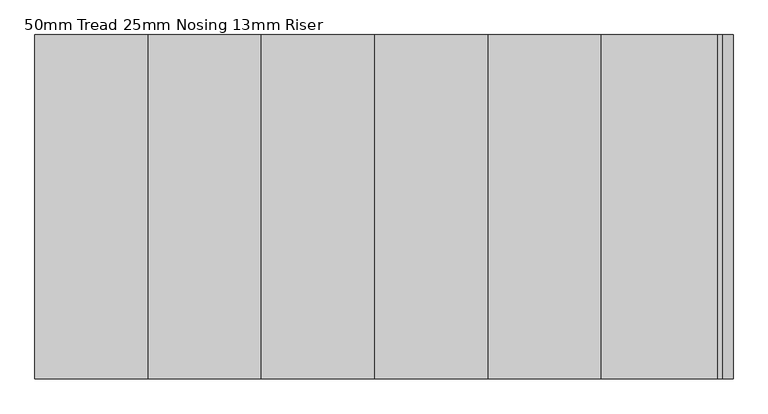
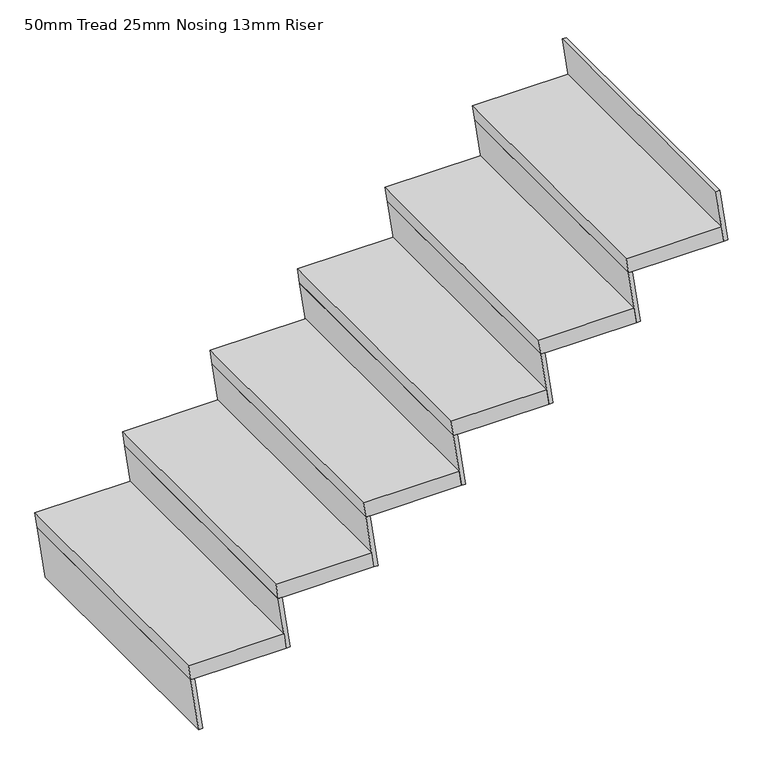
"""IFC4 building model written with IfcOpenShell, lengths in millimetres: stair flight geometry, 50mm Tread 25mm Nosing 13mm Riser."""

from ifc_helpers import new_model, si_unit, frame, origin, place, context, project, spatial, polyline, outline, extrude, source, transform, mapped, element, save


def stair_flight_50mm_tread_25mm_nosing_13mm_riser_89ce4123(model_context):
    return source(origin(), model_context, "Body", "SweptSolid", [
        extrude(outline(polyline([(1739.1304348, -8778.6870075), (1739.1304348, -9078.6870075), (1689.1304348, -9071.4995075), (1689.1304348, -8771.4995075), (1739.1304348, -8778.6870075)])), frame((0.0, 2408.8252453, 0.0), z_axis=(0.0, 1.0, 0.0), x_axis=(0.0, 0.0, 1.0)), (0.0, 0.0, 1.0), 835.4613281),
        extrude(outline(polyline([(1689.1304348, -9071.4995075), (1515.2173913, -9046.4995075), (1515.2173913, -9033.8710175), (1689.1304348, -9058.8710175), (1689.1304348, -9071.4995075)])), frame((0.0, 2408.8252453, 0.0), z_axis=(0.0, 1.0, 0.0), x_axis=(0.0, 0.0, 1.0)), (0.0, 0.0, 1.0), 835.4613281),
        extrude(outline(polyline([(1863.0434783, -8796.4995075), (1689.1304348, -8771.4995075), (1689.1304348, -8758.8710175), (1863.0434783, -8783.8710175), (1863.0434783, -8796.4995075)])), frame((0.0, 2408.8252453, 0.0), z_axis=(0.0, 1.0, 0.0), x_axis=(0.0, 0.0, 1.0)), (0.0, 0.0, 1.0), 835.4613281),
        extrude(outline(polyline([(1913.0434783, -8503.6870075), (1913.0434783, -8803.6870075), (1863.0434783, -8796.4995075), (1863.0434783, -8496.4995075), (1913.0434783, -8503.6870075)])), frame((0.0, 2408.8252453, 0.0), z_axis=(0.0, 1.0, 0.0), x_axis=(0.0, 0.0, 1.0)), (0.0, 0.0, 1.0), 835.4613281),
        extrude(outline(polyline([(2036.9565217, -8521.4995075), (1863.0434783, -8496.4995075), (1863.0434783, -8483.8710175), (2036.9565217, -8508.8710175), (2036.9565217, -8521.4995075)])), frame((0.0, 2408.8252453, 0.0), z_axis=(0.0, 1.0, 0.0), x_axis=(0.0, 0.0, 1.0)), (0.0, 0.0, 1.0), 835.4613281),
        extrude(outline(polyline([(2086.9565217, -8228.6870075), (2086.9565217, -8528.6870075), (2036.9565217, -8521.4995075), (2036.9565217, -8221.4995075), (2086.9565217, -8228.6870075)])), frame((0.0, 2408.8252453, 0.0), z_axis=(0.0, 1.0, 0.0), x_axis=(0.0, 0.0, 1.0)), (0.0, 0.0, 1.0), 835.4613281),
        extrude(outline(polyline([(2210.8695652, -8246.4995075), (2036.9565217, -8221.4995075), (2036.9565217, -8208.8710175), (2210.8695652, -8233.8710175), (2210.8695652, -8246.4995075)])), frame((0.0, 2408.8252453, 0.0), z_axis=(0.0, 1.0, 0.0), x_axis=(0.0, 0.0, 1.0)), (0.0, 0.0, 1.0), 835.4613281),
        extrude(outline(polyline([(2260.8695652, -7953.6870075), (2260.8695652, -8253.6870075), (2210.8695652, -8246.4995075), (2210.8695652, -7946.4995075), (2260.8695652, -7953.6870075)])), frame((0.0, 2408.8252453, 0.0), z_axis=(0.0, 1.0, 0.0), x_axis=(0.0, 0.0, 1.0)), (0.0, 0.0, 1.0), 835.4613281),
        extrude(outline(polyline([(2384.7826087, -7971.4995075), (2210.8695652, -7946.4995075), (2210.8695652, -7933.8710175), (2384.7826087, -7958.8710175), (2384.7826087, -7971.4995075)])), frame((0.0, 2408.8252453, 0.0), z_axis=(0.0, 1.0, 0.0), x_axis=(0.0, 0.0, 1.0)), (0.0, 0.0, 1.0), 835.4613281),
        extrude(outline(polyline([(2434.7826087, -7678.6870075), (2434.7826087, -7978.6870075), (2384.7826087, -7971.4995075), (2384.7826087, -7671.4995075), (2434.7826087, -7678.6870075)])), frame((0.0, 2408.8252453, 0.0), z_axis=(0.0, 1.0, 0.0), x_axis=(0.0, 0.0, 1.0)), (0.0, 0.0, 1.0), 835.4613281),
        extrude(outline(polyline([(2558.6956522, -7696.4995075), (2384.7826087, -7671.4995075), (2384.7826087, -7658.8710175), (2558.6956522, -7683.8710175), (2558.6956522, -7696.4995075)])), frame((0.0, 2408.8252453, 0.0), z_axis=(0.0, 1.0, 0.0), x_axis=(0.0, 0.0, 1.0)), (0.0, 0.0, 1.0), 835.4613281),
        extrude(outline(polyline([(2732.6086957, -7421.4995075), (2558.6956522, -7396.4995075), (2558.6956522, -7383.8710175), (2732.6086957, -7408.8710175), (2732.6086957, -7421.4995075)])), frame((0.0, 2408.8252453, 0.0), z_axis=(0.0, 1.0, 0.0), x_axis=(0.0, 0.0, 1.0)), (0.0, 0.0, 1.0), 835.4613281),
        extrude(outline(polyline([(2608.6956522, -7403.6870075), (2608.6956522, -7703.6870075), (2558.6956522, -7696.4995075), (2558.6956522, -7396.4995075), (2608.6956522, -7403.6870075)])), frame((0.0, 2408.8252453, 0.0), z_axis=(0.0, 1.0, 0.0), x_axis=(0.0, 0.0, 1.0)), (0.0, 0.0, 1.0), 835.4613281),
    ])


if __name__ == "__main__":
    model = new_model("IFC4")
    model_context = context("Model", 3, world=origin())
    ifc_project = project(units=[si_unit("LENGTHUNIT", "METRE", prefix="MILLI")], contexts=[model_context])
    site = spatial("IfcSite", under=ifc_project)
    building = spatial("IfcBuilding", under=site)
    placement = place(None, origin())
    stair_flight_50mm_tread_25mm_nosing_13mm_riser_shape = stair_flight_50mm_tread_25mm_nosing_13mm_riser_89ce4123(model_context)
    element("IfcStairFlight", 1, ObjectType="50mm Tread 25mm Nosing 13mm Riser", at=placement, inside=building, context=model_context, shape_type="MappedRepresentation", body=[
        mapped(stair_flight_50mm_tread_25mm_nosing_13mm_riser_shape, transform((0.0, 0.0, 0.0), x_axis=(1.0, 0.0, 0.0), y_axis=(0.0, 1.0, 0.0), z_axis=(0.0, 0.0, 1.0))),
    ])
    save(model, "model.ifc")
